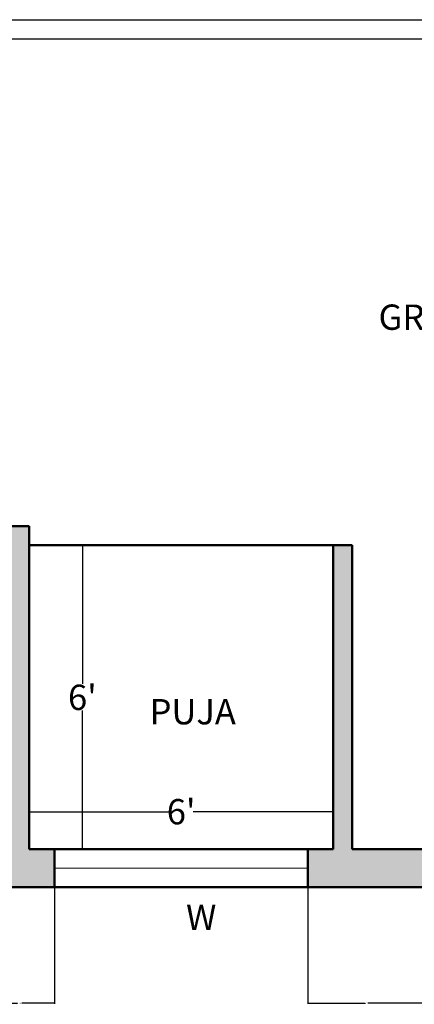
# Model space of a CAD drawing. Units: inches. Extents: x -22 to 470, y -437 to 97.
# Tile 3 of 9: x 211 to 304, y -425 to -192. Entities that reach past the tile are written whole.
import ezdxf

# ---------------------------------------------------------------- set-up
doc = ezdxf.new("R2010")
doc.units = ezdxf.units.IN
doc.header["$MEASUREMENT"] = 0
for name, color, linetype, lineweight in [('A-ANNO-DIMS', 2, 'Continuous', 18), ('A-ANNO-TEXT', 7, 'Continuous', 18), ('A-AREA-IDEN', 7, 'Continuous', 25), ('A-GLAZ', 4, 'Continuous', 18), ('A-WALL', 7, 'Continuous', 50), ('A-WALL-PATT', 8, 'Continuous', 13)]:
    doc.layers.add(name, color=color, linetype=linetype, lineweight=lineweight)
doc.styles.get("Standard").update_dxf_attribs({"font": 'arial.ttf'})
doc.dimstyles.get("Standard").update_dxf_attribs({"dimtxt": 0.18, "dimasz": 0.18, "dimexe": 0.18, "dimexo": 0.0625, "dimgap": 0.09, "dimtad": 0, "dimtih": 1, "dimtoh": 1, "dimdec": 0, "dimzin": 0, "dimdsep": 46, "dimlunit": 3, "dimtxsty": 'Standard', "dimcen": 0.09, "dimadec": 0, "dimazin": 0, "dimtfac": 1, "dimtdec": 0, "dimtofl": 0, "dimtmove": 0, "dimatfit": 3, "dimfxl": 1, "dimtolj": 1, "dimtzin": 0, "dimarcsym": 0})

# ---------------------------------------------------------------- blocks, each defined once
blk = doc.blocks.new('*D18')
at = {"layer": 'A-ANNO-DIMS', "color": 0, "lineweight": -2, "transparency": 16777216}
for p, q in [((225.52, -316.94), (225.52, -349.6)), ((225.58, -316.76), (225.7, -316.76)), ((225.52, -388.58), (225.52, -355.91)), ((225.58, -388.76), (225.7, -388.76))]:
    blk.add_line(p, q, dxfattribs=at)
at = {"layer": 'A-ANNO-DIMS', "color": 0, "transparency": 16777216}
for points in [[(225.49, -316.94), (225.55, -316.94), (225.52, -316.76)], [(225.49, -388.58), (225.55, -388.58), (225.52, -388.76)]]:
    blk.add_solid(points, dxfattribs=at)
at = {"layer": 'Defpoints', "color": 0, "transparency": 16777216}
for p in [(225.52, -316.76), (225.52, -388.76), (225.52, -388.76)]:
    blk.add_point(p, dxfattribs=at)
at = {"layer": 'A-ANNO-DIMS', "color": 0, "transparency": 16777216, "insert": (225.52, -352.76), "char_height": 6, "attachment_point": 5}
blk.add_mtext("\\A1;6'", dxfattribs=at)
blk = doc.blocks.new('*D19')
at = {"layer": 'A-ANNO-DIMS', "color": 0, "lineweight": -2, "transparency": 16777216}
for p, q in [((212.92, -377.95), (212.92, -380.03)), ((213.1, -379.85), (246.05, -379.85)), ((284.74, -379.85), (251.79, -379.85)), ((284.92, -377.95), (284.92, -380.03))]:
    blk.add_line(p, q, dxfattribs=at)
at = {"layer": 'A-ANNO-DIMS', "color": 0, "transparency": 16777216}
for points in [[(213.1, -379.82), (213.1, -379.88), (212.92, -379.85)], [(284.74, -379.82), (284.74, -379.88), (284.92, -379.85)]]:
    blk.add_solid(points, dxfattribs=at)
at = {"layer": 'Defpoints', "color": 0, "transparency": 16777216}
for p in [(212.92, -377.88), (284.92, -377.88), (284.92, -379.85)]:
    blk.add_point(p, dxfattribs=at)
at = {"layer": 'A-ANNO-DIMS', "color": 0, "transparency": 16777216, "insert": (248.92, -379.85), "char_height": 6, "attachment_point": 5}
blk.add_mtext("\\A1;6'", dxfattribs=at)
blk = doc.blocks.new('WINDOW-60-SASH')
for p, q in [((0, 9), (60, 9)), ((0, 4.5), (60, 4.5)), ((60, 0), (0, 0))]:
    blk.add_line(p, q)
blk = doc.blocks.new('*D64')
at = {"layer": 'A-ANNO-DIMS', "color": 0, "lineweight": -2, "transparency": 16777216}
for p, q in [((168.98, -192.26), (470.05, -192.26)), ((469.87, -192.44), (469.87, -194.32)), ((469.87, -196.58), (469.87, -194.69)), ((168.98, -196.76), (470.05, -196.76))]:
    blk.add_line(p, q, dxfattribs=at)
at = {"layer": 'A-ANNO-DIMS', "color": 0, "transparency": 16777216}
for points in [[(469.84, -192.44), (469.9, -192.44), (469.87, -192.26)], [(469.84, -196.58), (469.9, -196.58), (469.87, -196.76)]]:
    blk.add_solid(points, dxfattribs=at)
at = {"layer": 'Defpoints', "color": 0, "transparency": 16777216}
for p in [(168.92, -192.26), (168.92, -196.76), (469.87, -196.76)]:
    blk.add_point(p, dxfattribs=at)
at = {"layer": 'A-ANNO-DIMS', "color": 0, "transparency": 16777216, "insert": (469.87, -194.51), "char_height": 0.18, "attachment_point": 5}
blk.add_mtext('\\A1;0\'-4 1/2"', dxfattribs=at)
blk = doc.blocks.new('*D74')
at = {"layer": 'A-ANNO-DIMS', "color": 0, "lineweight": -2, "transparency": 16777216}
for p, q in [((202.42, -397.82), (202.42, -425.39)), ((218.92, -397.82), (218.92, -425.39)), ((202.6, -425.21), (210.14, -425.21)), ((218.74, -425.21), (211.2, -425.21))]:
    blk.add_line(p, q, dxfattribs=at)
at = {"layer": 'A-ANNO-DIMS', "color": 0, "transparency": 16777216}
for points in [[(202.6, -425.18), (202.6, -425.24), (202.42, -425.21)], [(218.74, -425.18), (218.74, -425.24), (218.92, -425.21)]]:
    blk.add_solid(points, dxfattribs=at)
at = {"layer": 'Defpoints', "color": 0, "transparency": 16777216}
for p in [(202.42, -397.76), (218.92, -397.76), (218.92, -425.21)]:
    blk.add_point(p, dxfattribs=at)
at = {"layer": 'A-ANNO-DIMS', "color": 0, "transparency": 16777216, "insert": (210.67, -425.21), "char_height": 0.18, "attachment_point": 5}
blk.add_mtext('\\A1;1\'-4 1/2"', dxfattribs=at)
blk = doc.blocks.new('*D75')
at = {"layer": 'A-ANNO-DIMS', "color": 0, "lineweight": -2, "transparency": 16777216}
for p, q in [((278.92, -397.82), (278.92, -425.39)), ((306.75, -397.82), (306.75, -425.39)), ((279.1, -425.21), (292.51, -425.21)), ((306.57, -425.21), (293.17, -425.21))]:
    blk.add_line(p, q, dxfattribs=at)
at = {"layer": 'A-ANNO-DIMS', "color": 0, "transparency": 16777216}
for points in [[(279.1, -425.18), (279.1, -425.24), (278.92, -425.21)], [(306.57, -425.18), (306.57, -425.24), (306.75, -425.21)]]:
    blk.add_solid(points, dxfattribs=at)
at = {"layer": 'Defpoints', "color": 0, "transparency": 16777216}
for p in [(278.92, -397.76), (306.75, -397.76), (306.75, -425.21)]:
    blk.add_point(p, dxfattribs=at)
at = {"layer": 'A-ANNO-DIMS', "color": 0, "transparency": 16777216, "insert": (292.84, -425.21), "char_height": 0.18, "attachment_point": 5}
blk.add_mtext('\\A1;2\'-4"', dxfattribs=at)

msp = doc.modelspace()

# ---------------------------------------------------------------- hatches: boundary and pattern name
at = {"layer": 'A-WALL-PATT'}
h = msp.add_hatch(color=256, dxfattribs=at)
h.dxf.hatch_style = 1
h.paths.add_polyline_path([(130.42, 13.24), (26.92, 13.24), (26.92, -43.76), (35.92, -43.76), (35.92, 4.24), (83.92, 4.24), (83.92, 1.24), (88.42, 1.24), (88.42, 4.24), (130.42, 4.24)])
h.paths.add_polyline_path([(266.92, 13.24), (190.42, 13.24), (190.42, 4.24), (232.42, 4.24), (232.42, -115.76), (229.42, -115.76), (229.42, -120.26), (239.92, -120.26), (239.92, -115.76), (236.92, -115.76), (236.92, 4.24), (266.92, 4.24)])
h.paths.add_polyline_path([(442.42, 13.24), (326.92, 13.24), (326.92, 4.24), (356.92, 4.24), (356.92, 1.24), (361.42, 1.24), (361.42, 4.24), (433.42, 4.24), (433.42, -49.38), (442.42, -49.38)])
h.paths.add_polyline_path([(442.42, -73.38), (433.42, -73.38), (433.42, -115.76), (361.42, -115.76), (361.42, -22.76), (356.92, -22.76), (356.92, -115.76), (263.92, -115.76), (263.92, -120.26), (332.92, -120.26), (332.92, -123.26), (337.42, -123.26), (337.42, -120.26), (433.42, -120.26), (433.42, -148.49), (442.42, -148.49)])
h.paths.add_polyline_path([(205.42, -115.76), (88.42, -115.76), (88.42, -22.76), (83.92, -22.76), (83.92, -115.76), (35.92, -115.76), (35.92, -67.76), (26.92, -67.76), (26.92, -126.26), (35.92, -126.26), (35.92, -120.26), (205.42, -120.26)])
h.paths.add_polyline_path([(35.92, -196.76), (168.92, -196.76), (168.92, -192.26), (35.92, -192.26), (35.92, -186.26), (26.92, -186.26), (26.92, -224.25), (35.92, -224.25)])
h.paths.add_polyline_path([(35.92, -284.25), (26.92, -284.25), (26.92, -397.76), (53.92, -397.76), (53.92, -388.76), (35.92, -388.76)])
h.paths.add_polyline_path([(142.42, -388.76), (136.42, -388.76), (136.42, -316.76), (181.42, -316.76), (181.42, -312.26), (136.42, -312.26), (136.42, -303.75), (131.92, -303.75), (131.92, -388.76), (113.92, -388.76), (113.92, -397.76), (142.42, -397.76)])
h.paths.add_polyline_path([(218.92, -388.76), (212.92, -388.76), (212.92, -312.26), (205.42, -312.26), (205.42, -316.76), (208.42, -316.76), (208.42, -388.76), (202.42, -388.76), (202.42, -397.76), (218.92, -397.76)])
h.paths.add_polyline_path([(306.75, -388.76), (289.42, -388.76), (289.42, -316.76), (284.92, -316.76), (284.92, -388.76), (278.92, -388.76), (278.92, -397.76), (306.75, -397.76)])
h.paths.add_polyline_path([(391.42, -388.76), (366.75, -388.76), (366.75, -397.76), (391.42, -397.76)], flags=17)
h.paths.add_polyline_path([(442.42, -172.49), (433.42, -172.49), (433.42, -192.26), (337.42, -192.26), (337.42, -147.26), (332.92, -147.26), (332.92, -196.76), (433.42, -196.76), (433.42, -388.76), (427.42, -388.76), (427.42, -397.76), (442.42, -397.76)])

# ---------------------------------------------------------------- linework, layer by layer
at = {"layer": 'A-WALL'}
for p, q in [((136.42, -312.26), (212.92, -312.26)), ((212.92, -312.26), (212.92, -388.76)), ((212.92, -316.76), (289.42, -316.76)), ((284.92, -316.76), (284.92, -388.76)), ((289.42, -316.76), (289.42, -388.76)), ((212.92, -388.76), (284.92, -388.76)), ((218.92, -397.76), (218.92, -388.76)), ((278.92, -388.76), (278.92, -397.76)), ((289.42, -388.76), (391.42, -388.76)), ((26.92, -397.76), (391.42, -397.76))]:
    msp.add_line(p, q, dxfattribs=at)

# ---------------------------------------------------------------- block references
at = {"layer": 'A-GLAZ'}
msp.add_blockref('WINDOW-60-SASH', (218.92, -397.76), dxfattribs=at)

# ---------------------------------------------------------------- texts
at = {"layer": 'A-ANNO-TEXT', "insert": (250.08, -401.84), "char_height": 6, "attachment_point": 1}
msp.add_mtext('W', dxfattribs=at)
at = {"layer": 'A-AREA-IDEN', "char_height": 6, "attachment_point": 1}
for s, insert in [('GREAT ROOM', (295.68, -259.72)), ('PUJA', (241.44, -353.17))]:
    msp.add_mtext(s, dxfattribs=dict(at, insert=insert))

# ---------------------------------------------------------------- dimensions: what is measured, and where the dimension line sits
at = {"layer": 'A-ANNO-DIMS'}
for base, p1, p2, override, picture, middle in [((469.87, -196.76), (168.92, -192.26), (168.92, -196.76), {"dimdec": 1, "dimlfac": 1, "dimrnd": 0, "dimzin": 1, "dimdsep": 46, "dimlunit": 4, "dimfrac": 2}, '*D64', (469.87, -194.51)), ((225.52, -388.76), (225.52, -316.76), (225.52, -388.76), {"dimtxt": 6, "dimclrd": 0, "dimclre": 0, "dimclrt": 0}, '*D18', (225.52, -352.76))]:
    dim = msp.add_linear_dim(base=base, p1=p1, p2=p2, angle=90, dimstyle='Standard', override=override, dxfattribs=at)
    dim.commit()
    dim.dimension.update_dxf_attribs({"geometry": picture, "text_midpoint": middle})
for base, p1, p2, override, picture, middle in [((284.92, -379.85), (212.92, -377.88), (284.92, -377.88), {"dimtxt": 6, "dimclrd": 0, "dimclre": 0, "dimclrt": 0}, '*D19', (248.92, -379.85)), ((218.92, -425.21), (202.42, -397.76), (218.92, -397.76), {"dimdec": 1, "dimlfac": 1, "dimrnd": 0, "dimzin": 1, "dimdsep": 46, "dimlunit": 4, "dimfrac": 2}, '*D74', (210.67, -425.21)), ((306.75, -425.21), (278.92, -397.76), (306.75, -397.76), {"dimdec": 1, "dimlfac": 1, "dimrnd": 0, "dimzin": 1, "dimdsep": 46, "dimlunit": 4, "dimfrac": 2}, '*D75', (292.84, -425.21))]:
    dim = msp.add_linear_dim(base=base, p1=p1, p2=p2, dimstyle='Standard', override=override, dxfattribs=at)
    dim.commit()
    dim.dimension.update_dxf_attribs({"geometry": picture, "text_midpoint": middle})

doc.saveas('drawing.dxf')
